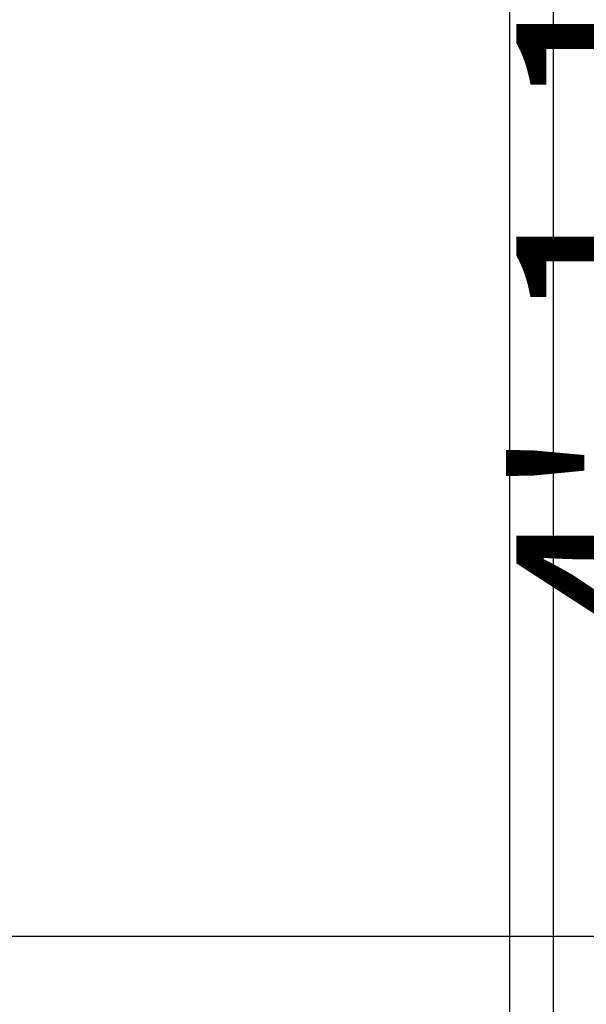
# Model space of a CAD drawing. Units: inches. Extents: x 459864 to 460310, y 324185 to 324787.
# Tile 106 of 112: x 460255 to 460272, y 324281 to 324311. Entities that reach past the tile are written whole.
import ezdxf

# ---------------------------------------------------------------- set-up
doc = ezdxf.new("R2010")
doc.units = ezdxf.units.IN
for name, color, linetype, lineweight in [('A-ANNO-DIMS', 2, 'Continuous', 18), ('C-PROP', 7, 'Continuous', 30), ('L-HRDS', 9, 'Continuous', 18), ('L-SITE-PATT', 252, 'Continuous', 13)]:
    doc.layers.add(name, color=color, linetype=linetype, lineweight=lineweight)
doc.styles.get("Standard").update_dxf_attribs({"font": 'arial.ttf'})
doc.dimstyles.new('ISO-25', dxfattribs={"dimtxt": 6, "dimasz": 2.5, "dimexe": 1.25, "dimexo": 0.625, "dimtad": 1, "dimdec": 1, "dimlunit": 3, "dimtxsty": 'Standard', "dimcen": 2.5, "dimadec": 0, "dimazin": 0, "dimtfac": 1, "dimtdec": 1, "dimtmove": 0, "dimatfit": 3, "dimfxl": 1, "dimarcsym": 0})

# ---------------------------------------------------------------- blocks, each defined once
blk = doc.blocks.new('*D21')
at = {"layer": 'A-ANNO-DIMS', "color": 0, "lineweight": -2, "transparency": 16777216}
for p, q in [((460247.74, 324715.483), (460309.58, 324715.483)), ((460308.33, 324712.983), (460308.33, 324285.983)), ((460247.74, 324283.483), (460309.58, 324283.483))]:
    blk.add_line(p, q, dxfattribs=at)
at = {"layer": 'A-ANNO-DIMS', "color": 0, "transparency": 16777216}
for points in [[(460307.914, 324712.983), (460308.747, 324712.983), (460308.33, 324715.483)], [(460307.914, 324285.983), (460308.747, 324285.983), (460308.33, 324283.483)]]:
    blk.add_solid(points, dxfattribs=at)
at = {"layer": 'Defpoints', "color": 0, "transparency": 16777216}
for p in [(460247.115, 324715.483), (460247.115, 324283.483), (460308.33, 324283.483)]:
    blk.add_point(p, dxfattribs=at)
at = {"layer": 'A-ANNO-DIMS', "color": 0, "transparency": 16777216, "insert": (460304.64, 324499.483), "char_height": 6, "attachment_point": 5, "rotation": 90}
blk.add_mtext("36'", dxfattribs=at)
blk = doc.blocks.new('*D62')
at = {"layer": 'A-ANNO-DIMS', "color": 0, "lineweight": -2, "transparency": 16777216}
for p, q in [((460247.74, 324332.739), (460278.765, 324332.739)), ((460277.515, 324330.239), (460277.515, 324285.983)), ((460247.74, 324283.483), (460278.765, 324283.483))]:
    blk.add_line(p, q, dxfattribs=at)
at = {"layer": 'A-ANNO-DIMS', "color": 0, "transparency": 16777216}
for points in [[(460277.098, 324330.239), (460277.932, 324330.239), (460277.515, 324332.739)], [(460277.098, 324285.983), (460277.932, 324285.983), (460277.515, 324283.483)]]:
    blk.add_solid(points, dxfattribs=at)
at = {"layer": 'Defpoints', "color": 0, "transparency": 16777216}
for p in [(460247.115, 324332.739), (460247.115, 324283.483), (460277.515, 324283.483)]:
    blk.add_point(p, dxfattribs=at)
at = {"layer": 'A-ANNO-DIMS', "color": 0, "transparency": 16777216, "insert": (460273.788, 324308.111), "char_height": 6, "attachment_point": 5, "rotation": 90}
blk.add_mtext('4\'-1 1/2"', dxfattribs=at)
blk = doc.blocks.new('*D65')
at = {"layer": 'A-ANNO-DIMS', "color": 0, "lineweight": -2, "transparency": 16777216}
for p, q in [((460247.74, 324283.483), (460302.765, 324283.483)), ((460301.515, 324280.983), (460301.515, 324197.483)), ((460271.74, 324194.983), (460302.765, 324194.983))]:
    blk.add_line(p, q, dxfattribs=at)
at = {"layer": 'A-ANNO-DIMS', "color": 0, "transparency": 16777216}
for points in [[(460301.098, 324280.983), (460301.932, 324280.983), (460301.515, 324283.483)], [(460301.098, 324197.483), (460301.932, 324197.483), (460301.515, 324194.983)]]:
    blk.add_solid(points, dxfattribs=at)
at = {"layer": 'Defpoints', "color": 0, "transparency": 16777216}
for p in [(460247.115, 324283.483), (460271.115, 324194.983), (460301.515, 324194.983)]:
    blk.add_point(p, dxfattribs=at)
at = {"layer": 'A-ANNO-DIMS', "color": 0, "transparency": 16777216, "insert": (460297.788, 324239.233), "char_height": 6, "attachment_point": 5, "rotation": 90}
blk.add_mtext('7\'-4 1/2"', dxfattribs=at)

msp = doc.modelspace()

# ---------------------------------------------------------------- hatches: boundary and pattern name
at = {"layer": 'L-SITE-PATT'}
h = msp.add_hatch(dxfattribs=at)
h.set_pattern_fill('DOTS', color=256)
h.paths.add_polyline_path([(460269.804, 324283.483), (460247.115, 324283.483), (460121.929, 324283.483), (460121.929, 324252.473), (460117.429, 324252.473), (460110.124, 324252.473), (460110.124, 324243.287), (460080.83, 324243.287), (460080.83, 324252.473), (460061.115, 324252.473), (460061.115, 324251.882), (460077.909, 324251.882), (460077.909, 324199.483), (460080.83, 324199.483), (460080.83, 324207.553), (460110.124, 324207.553), (460110.124, 324199.483), (460110.813, 324199.483), (460262.115, 324199.483), (460269.804, 324199.483)], flags=17)
edge = h.paths.add_edge_path(flags=0)
edge.add_ellipse((460222.59, 324263.813), major_axis=(-8.485, 8.485), ratio=1, start_angle=405, end_angle=495, ccw=False)
edge.add_line((460214.821, 324254.66), (460214.832, 324254.666))
edge.add_ellipse((460222.59, 324263.813), major_axis=(-8.485, 8.485), ratio=1, start_angle=405, end_angle=495, ccw=False)
edge.add_line((460210.759, 324261.781), (460210.768, 324261.787))
edge.add_ellipse((460222.59, 324263.813), major_axis=(-8.485, 8.485), ratio=1, start_angle=405, end_angle=495, ccw=False)
edge.add_ellipse((460222.59, 324263.813), major_axis=(-8.485, 8.485), ratio=1, start_angle=392.754, end_angle=405, ccw=False)
edge.add_ellipse((460222.59, 324263.813), major_axis=(-8.485, 8.485), ratio=1, start_angle=380.9347, end_angle=392.754, ccw=False)
edge.add_line((460211.337, 324267.985), (460211.34, 324267.985))
edge.add_ellipse((460222.59, 324263.813), major_axis=(-8.485, 8.485), ratio=1, start_angle=380.9347, end_angle=392.754, ccw=False)
edge.add_ellipse((460222.59, 324263.813), major_axis=(-8.485, 8.485), ratio=1, start_angle=347.9015, end_angle=380.9347, ccw=False)
edge.add_ellipse((460222.59, 324263.813), major_axis=(-8.485, 8.485), ratio=1, start_angle=327.0619, end_angle=347.9015, ccw=False)
edge.add_ellipse((460222.59, 324263.813), major_axis=(-8.485, 8.485), ratio=1, start_angle=278.3246, end_angle=327.0619, ccw=False)
edge.add_line((460225.158, 324275.536), (460225.158, 324275.535))
edge.add_ellipse((460222.59, 324263.813), major_axis=(-8.485, 8.485), ratio=1, start_angle=278.3246, end_angle=327.0619, ccw=False)
edge.add_ellipse((460222.59, 324263.813), major_axis=(-8.485, 8.485), ratio=1, start_angle=260.6436, end_angle=278.3246, ccw=False)
edge.add_ellipse((460222.59, 324263.813), major_axis=(-8.485, 8.485), ratio=1, start_angle=225, end_angle=260.6436, ccw=False)
edge.add_line((460234.509, 324265.243), (460234.501, 324265.239))
edge.add_ellipse((460222.59, 324263.813), major_axis=(-8.485, 8.485), ratio=1, start_angle=225, end_angle=260.6436, ccw=False)
edge.add_ellipse((460222.59, 324263.813), major_axis=(-8.485, 8.485), ratio=1, start_angle=495, end_angle=585, ccw=False)
edge.add_line((460234.437, 324261.861), (460234.424, 324261.858))
edge.add_ellipse((460222.59, 324263.813), major_axis=(-8.485, 8.485), ratio=1, start_angle=495, end_angle=585, ccw=False)
edge.add_line((460227.95, 324253.067), (460227.946, 324253.083))
edge.add_ellipse((460222.59, 324263.813), major_axis=(-8.485, 8.485), ratio=1, start_angle=495, end_angle=585, ccw=False)
edge.add_line((460226.223, 324252.369), (460226.211, 324252.38))
edge.add_ellipse((460222.59, 324263.813), major_axis=(-8.485, 8.485), ratio=1, start_angle=495, end_angle=585, ccw=False)
h.paths.add_polyline_path([(460219.651, 324254.347), (460218.461, 324253.545), (460218.275, 324254.789), (460219.642, 324256.542), (460219.625, 324260.848), (460216.11, 324257.333), (460214.35, 324256.978), (460215.416, 324259.356), (460212.524, 324258.496), (460213.137, 324259.93), (460218.507, 324263.813), (460222.59, 324263.813), (460222.59, 324267.807), (460218.176, 324272.212), (460219.026, 324274.639), (460222.59, 324272.811), (460222.59, 324275.423), (460223.057, 324274.825), (460222.675, 324273.492), (460225.912, 324267.135), (460219.625, 324260.848)], flags=0)
edge = h.paths.add_edge_path(flags=0)
edge.add_ellipse((460194.576, 324264.046), major_axis=(-8.485, 8.485), ratio=1, start_angle=495, end_angle=585, ccw=False)
edge.add_line((460199.936, 324253.3), (460199.932, 324253.316))
edge.add_ellipse((460194.576, 324264.046), major_axis=(-8.485, 8.485), ratio=1, start_angle=495, end_angle=585, ccw=False)
edge.add_line((460198.208, 324252.603), (460198.196, 324252.613))
edge.add_ellipse((460194.576, 324264.046), major_axis=(-8.485, 8.485), ratio=1, start_angle=495, end_angle=585, ccw=False)
edge.add_ellipse((460194.576, 324264.046), major_axis=(-8.485, 8.485), ratio=1, start_angle=405, end_angle=495, ccw=False)
edge.add_line((460186.806, 324254.893), (460186.817, 324254.899))
edge.add_ellipse((460194.576, 324264.046), major_axis=(-8.485, 8.485), ratio=1, start_angle=405, end_angle=495, ccw=False)
edge.add_line((460182.744, 324262.014), (460182.753, 324262.02))
edge.add_ellipse((460194.576, 324264.046), major_axis=(-8.485, 8.485), ratio=1, start_angle=405, end_angle=495, ccw=False)
edge.add_ellipse((460194.576, 324264.046), major_axis=(-8.485, 8.485), ratio=1, start_angle=392.754, end_angle=405, ccw=False)
edge.add_ellipse((460194.576, 324264.046), major_axis=(-8.485, 8.485), ratio=1, start_angle=380.9347, end_angle=392.754, ccw=False)
edge.add_line((460183.323, 324268.218), (460183.326, 324268.218))
edge.add_ellipse((460194.576, 324264.046), major_axis=(-8.485, 8.485), ratio=1, start_angle=380.9347, end_angle=392.754, ccw=False)
edge.add_ellipse((460194.576, 324264.046), major_axis=(-8.485, 8.485), ratio=1, start_angle=347.9015, end_angle=380.9347, ccw=False)
edge.add_ellipse((460194.576, 324264.046), major_axis=(-8.485, 8.485), ratio=1, start_angle=327.0619, end_angle=347.9015, ccw=False)
edge.add_ellipse((460194.576, 324264.046), major_axis=(-8.485, 8.485), ratio=1, start_angle=278.3246, end_angle=327.0619, ccw=False)
edge.add_line((460197.144, 324275.769), (460197.143, 324275.768))
edge.add_ellipse((460194.576, 324264.046), major_axis=(-8.485, 8.485), ratio=1, start_angle=278.3246, end_angle=327.0619, ccw=False)
edge.add_ellipse((460194.576, 324264.046), major_axis=(-8.485, 8.485), ratio=1, start_angle=260.6436, end_angle=278.3246, ccw=False)
edge.add_ellipse((460194.576, 324264.046), major_axis=(-8.485, 8.485), ratio=1, start_angle=225, end_angle=260.6436, ccw=False)
edge.add_line((460206.494, 324265.476), (460206.487, 324265.473))
edge.add_ellipse((460194.576, 324264.046), major_axis=(-8.485, 8.485), ratio=1, start_angle=225, end_angle=260.6436, ccw=False)
edge.add_ellipse((460194.576, 324264.046), major_axis=(-8.485, 8.485), ratio=1, start_angle=495, end_angle=585, ccw=False)
edge.add_line((460206.422, 324262.094), (460206.409, 324262.091))
h.paths.add_polyline_path([(460191.61, 324261.081), (460191.637, 324254.58), (460190.447, 324253.778), (460190.261, 324255.023), (460191.628, 324256.775), (460191.61, 324261.081), (460188.096, 324257.566), (460186.335, 324257.211), (460187.402, 324259.589), (460184.509, 324258.729), (460185.123, 324260.163), (460190.493, 324264.046), (460194.576, 324264.046), (460194.576, 324268.04), (460190.161, 324272.446), (460191.011, 324274.872), (460194.576, 324273.044), (460194.576, 324275.657), (460195.043, 324275.058), (460194.661, 324273.725), (460197.897, 324267.368)], flags=0)
edge = h.paths.add_edge_path(flags=0)
edge.add_ellipse((460252.912, 324263.578), major_axis=(-8.485, 8.485), ratio=1, start_angle=405, end_angle=495, ccw=False)
edge.add_line((460241.081, 324261.545), (460241.089, 324261.551))
edge.add_ellipse((460252.912, 324263.578), major_axis=(-8.485, 8.485), ratio=1, start_angle=405, end_angle=495, ccw=False)
edge.add_ellipse((460252.912, 324263.578), major_axis=(-8.485, 8.485), ratio=1, start_angle=392.754, end_angle=405, ccw=False)
edge.add_ellipse((460252.912, 324263.578), major_axis=(-8.485, 8.485), ratio=1, start_angle=380.9347, end_angle=392.754, ccw=False)
edge.add_line((460241.659, 324267.749), (460241.662, 324267.749))
edge.add_ellipse((460252.912, 324263.578), major_axis=(-8.485, 8.485), ratio=1, start_angle=380.9347, end_angle=392.754, ccw=False)
edge.add_ellipse((460252.912, 324263.578), major_axis=(-8.485, 8.485), ratio=1, start_angle=347.9015, end_angle=380.9347, ccw=False)
edge.add_ellipse((460252.912, 324263.578), major_axis=(-8.485, 8.485), ratio=1, start_angle=327.0619, end_angle=347.9015, ccw=False)
edge.add_ellipse((460252.912, 324263.578), major_axis=(-8.485, 8.485), ratio=1, start_angle=278.3246, end_angle=327.0619, ccw=False)
edge.add_line((460255.48, 324275.3), (460255.479, 324275.299))
edge.add_ellipse((460252.912, 324263.578), major_axis=(-8.485, 8.485), ratio=1, start_angle=278.3246, end_angle=327.0619, ccw=False)
edge.add_ellipse((460252.912, 324263.578), major_axis=(-8.485, 8.485), ratio=1, start_angle=260.6436, end_angle=278.3246, ccw=False)
edge.add_ellipse((460252.912, 324263.578), major_axis=(-8.485, 8.485), ratio=1, start_angle=225, end_angle=260.6436, ccw=False)
edge.add_line((460264.83, 324265.007), (460264.823, 324265.004))
edge.add_ellipse((460252.912, 324263.578), major_axis=(-8.485, 8.485), ratio=1, start_angle=225, end_angle=260.6436, ccw=False)
edge.add_ellipse((460252.912, 324263.578), major_axis=(-8.485, 8.485), ratio=1, start_angle=495, end_angle=585, ccw=False)
edge.add_line((460264.758, 324261.626), (460264.745, 324261.622))
edge.add_ellipse((460252.912, 324263.578), major_axis=(-8.485, 8.485), ratio=1, start_angle=495, end_angle=585, ccw=False)
edge.add_line((460258.272, 324252.832), (460258.268, 324252.848))
edge.add_ellipse((460252.912, 324263.578), major_axis=(-8.485, 8.485), ratio=1, start_angle=495, end_angle=585, ccw=False)
edge.add_line((460256.545, 324252.134), (460256.533, 324252.144))
edge.add_ellipse((460252.912, 324263.578), major_axis=(-8.485, 8.485), ratio=1, start_angle=495, end_angle=585, ccw=False)
edge.add_ellipse((460252.912, 324263.578), major_axis=(-8.485, 8.485), ratio=1, start_angle=405, end_angle=495, ccw=False)
edge.add_line((460245.143, 324254.424), (460245.153, 324254.43))
h.paths.add_polyline_path([(460244.672, 324256.742), (460245.738, 324259.12), (460242.846, 324258.26), (460243.459, 324259.694), (460248.829, 324263.578), (460252.912, 324263.578), (460252.912, 324267.571), (460248.497, 324271.977), (460249.348, 324274.403), (460252.912, 324272.576), (460252.912, 324275.188), (460253.379, 324274.589), (460252.997, 324273.257), (460256.233, 324266.899), (460249.946, 324260.612), (460249.973, 324254.111), (460248.783, 324253.309), (460248.597, 324254.554), (460249.964, 324256.306), (460249.946, 324260.612), (460246.432, 324257.097)], flags=0)
edge = h.paths.add_edge_path(flags=0)
edge.add_ellipse((460167.439, 324262.833), major_axis=(-8.485, 8.485), ratio=1, start_angle=495, end_angle=585, ccw=False)
edge.add_line((460172.799, 324252.087), (460172.795, 324252.103))
edge.add_ellipse((460167.439, 324262.833), major_axis=(-8.485, 8.485), ratio=1, start_angle=495, end_angle=585, ccw=False)
edge.add_line((460171.071, 324251.389), (460171.059, 324251.399))
edge.add_ellipse((460167.439, 324262.833), major_axis=(-8.485, 8.485), ratio=1, start_angle=495, end_angle=585, ccw=False)
edge.add_ellipse((460167.439, 324262.833), major_axis=(-8.485, 8.485), ratio=1, start_angle=405, end_angle=495, ccw=False)
edge.add_line((460159.669, 324253.679), (460159.68, 324253.685))
edge.add_ellipse((460167.439, 324262.833), major_axis=(-8.485, 8.485), ratio=1, start_angle=405, end_angle=495, ccw=False)
edge.add_line((460155.607, 324260.8), (460155.616, 324260.806))
edge.add_ellipse((460167.439, 324262.833), major_axis=(-8.485, 8.485), ratio=1, start_angle=405, end_angle=495, ccw=False)
edge.add_ellipse((460167.439, 324262.833), major_axis=(-8.485, 8.485), ratio=1, start_angle=392.754, end_angle=405, ccw=False)
edge.add_ellipse((460167.439, 324262.833), major_axis=(-8.485, 8.485), ratio=1, start_angle=380.9347, end_angle=392.754, ccw=False)
edge.add_line((460156.185, 324267.005), (460156.189, 324267.005))
edge.add_ellipse((460167.439, 324262.833), major_axis=(-8.485, 8.485), ratio=1, start_angle=380.9347, end_angle=392.754, ccw=False)
edge.add_ellipse((460167.439, 324262.833), major_axis=(-8.485, 8.485), ratio=1, start_angle=347.9015, end_angle=380.9347, ccw=False)
edge.add_ellipse((460167.439, 324262.833), major_axis=(-8.485, 8.485), ratio=1, start_angle=327.0619, end_angle=347.9015, ccw=False)
edge.add_ellipse((460167.439, 324262.833), major_axis=(-8.485, 8.485), ratio=1, start_angle=278.3246, end_angle=327.0619, ccw=False)
edge.add_line((460170.007, 324274.556), (460170.006, 324274.554))
edge.add_ellipse((460167.439, 324262.833), major_axis=(-8.485, 8.485), ratio=1, start_angle=278.3246, end_angle=327.0619, ccw=False)
edge.add_ellipse((460167.439, 324262.833), major_axis=(-8.485, 8.485), ratio=1, start_angle=260.6436, end_angle=278.3246, ccw=False)
edge.add_ellipse((460167.439, 324262.833), major_axis=(-8.485, 8.485), ratio=1, start_angle=225, end_angle=260.6436, ccw=False)
edge.add_line((460179.357, 324264.262), (460179.35, 324264.259))
edge.add_ellipse((460167.439, 324262.833), major_axis=(-8.485, 8.485), ratio=1, start_angle=225, end_angle=260.6436, ccw=False)
edge.add_ellipse((460167.439, 324262.833), major_axis=(-8.485, 8.485), ratio=1, start_angle=495, end_angle=585, ccw=False)
edge.add_line((460179.285, 324260.881), (460179.272, 324260.877))
h.paths.add_polyline_path([(460164.473, 324259.867), (460164.5, 324253.366), (460163.31, 324252.565), (460163.124, 324253.809), (460164.491, 324255.561), (460164.473, 324259.867), (460160.958, 324256.353), (460159.198, 324255.998), (460160.265, 324258.375), (460157.372, 324257.515), (460157.986, 324258.949), (460163.356, 324262.833), (460167.439, 324262.833), (460167.439, 324266.826), (460163.024, 324271.232), (460163.874, 324273.659), (460167.439, 324271.831), (460167.439, 324274.443), (460167.905, 324273.844), (460167.524, 324272.512), (460170.76, 324266.154)], flags=0)
edge = h.paths.add_edge_path(flags=0)
edge.add_ellipse((460140.758, 324262.37), major_axis=(-8.485, 8.485), ratio=1, start_angle=495, end_angle=585, ccw=False)
edge.add_line((460146.118, 324251.624), (460146.114, 324251.639))
edge.add_ellipse((460140.758, 324262.37), major_axis=(-8.485, 8.485), ratio=1, start_angle=495, end_angle=585, ccw=False)
edge.add_line((460144.391, 324250.926), (460144.379, 324250.936))
edge.add_ellipse((460140.758, 324262.37), major_axis=(-8.485, 8.485), ratio=1, start_angle=495, end_angle=585, ccw=False)
edge.add_ellipse((460140.758, 324262.37), major_axis=(-8.485, 8.485), ratio=1, start_angle=405, end_angle=495, ccw=False)
edge.add_line((460132.989, 324253.216), (460132.999, 324253.222))
edge.add_ellipse((460140.758, 324262.37), major_axis=(-8.485, 8.485), ratio=1, start_angle=405, end_angle=495, ccw=False)
edge.add_line((460128.927, 324260.337), (460128.935, 324260.343))
edge.add_ellipse((460140.758, 324262.37), major_axis=(-8.485, 8.485), ratio=1, start_angle=405, end_angle=495, ccw=False)
edge.add_ellipse((460140.758, 324262.37), major_axis=(-8.485, 8.485), ratio=1, start_angle=392.754, end_angle=405, ccw=False)
edge.add_ellipse((460140.758, 324262.37), major_axis=(-8.485, 8.485), ratio=1, start_angle=380.9347, end_angle=392.754, ccw=False)
edge.add_line((460129.505, 324266.541), (460129.508, 324266.541))
edge.add_ellipse((460140.758, 324262.37), major_axis=(-8.485, 8.485), ratio=1, start_angle=380.9347, end_angle=392.754, ccw=False)
edge.add_ellipse((460140.758, 324262.37), major_axis=(-8.485, 8.485), ratio=1, start_angle=347.9015, end_angle=380.9347, ccw=False)
edge.add_ellipse((460140.758, 324262.37), major_axis=(-8.485, 8.485), ratio=1, start_angle=327.0619, end_angle=347.9015, ccw=False)
edge.add_ellipse((460140.758, 324262.37), major_axis=(-8.485, 8.485), ratio=1, start_angle=278.3246, end_angle=327.0619, ccw=False)
edge.add_line((460143.326, 324274.092), (460143.325, 324274.091))
edge.add_ellipse((460140.758, 324262.37), major_axis=(-8.485, 8.485), ratio=1, start_angle=278.3246, end_angle=327.0619, ccw=False)
edge.add_ellipse((460140.758, 324262.37), major_axis=(-8.485, 8.485), ratio=1, start_angle=260.6436, end_angle=278.3246, ccw=False)
edge.add_ellipse((460140.758, 324262.37), major_axis=(-8.485, 8.485), ratio=1, start_angle=225, end_angle=260.6436, ccw=False)
edge.add_line((460152.677, 324263.799), (460152.669, 324263.796))
edge.add_ellipse((460140.758, 324262.37), major_axis=(-8.485, 8.485), ratio=1, start_angle=225, end_angle=260.6436, ccw=False)
edge.add_ellipse((460140.758, 324262.37), major_axis=(-8.485, 8.485), ratio=1, start_angle=495, end_angle=585, ccw=False)
edge.add_line((460152.604, 324260.418), (460152.592, 324260.414))
h.paths.add_polyline_path([(460137.792, 324259.404), (460137.819, 324252.903), (460136.629, 324252.101), (460136.443, 324253.346), (460137.81, 324255.098), (460137.792, 324259.404), (460134.278, 324255.889), (460132.518, 324255.534), (460133.584, 324257.912), (460130.692, 324257.052), (460131.305, 324258.486), (460136.675, 324262.37), (460140.758, 324262.37), (460140.758, 324266.363), (460136.343, 324270.769), (460137.194, 324273.195), (460140.758, 324271.367), (460140.758, 324273.98), (460141.225, 324273.381), (460140.843, 324272.049), (460144.079, 324265.691)], flags=0)
h.paths.add_polyline_path([(460110.124, 324227.414), (460080.83, 324227.414), (460080.83, 324235.484), (460110.124, 324235.484)], flags=16)
h.paths.add_polyline_path([(460110.124, 324220.797), (460110.124, 324212.727), (460080.83, 324212.727), (460080.83, 324220.797)], flags=16)
h.paths.add_polyline_path([(460269.804, 324283.483), (460247.115, 324283.483), (460121.929, 324283.483), (460121.929, 324252.473), (460117.429, 324252.473), (460110.124, 324252.473), (460110.124, 324243.287), (460080.83, 324243.287), (460080.83, 324252.473), (460061.115, 324252.473), (460061.115, 324251.882), (460077.909, 324251.882), (460077.909, 324199.483), (460080.83, 324199.483), (460080.83, 324207.553), (460110.124, 324207.553), (460110.124, 324199.483), (460262.115, 324199.483), (460269.804, 324199.483)], flags=17)
h.paths.add_polyline_path([(460219.651, 324254.347), (460218.461, 324253.545), (460218.275, 324254.789), (460219.642, 324256.542), (460219.625, 324260.848), (460216.11, 324257.333), (460214.35, 324256.978), (460215.416, 324259.356), (460212.524, 324258.496), (460213.137, 324259.93), (460218.507, 324263.813), (460222.59, 324263.813), (460220.18, 324266.223), (460215.461, 324265.308), (460211.835, 324266.137), (460216.247, 324267.985), (460218.418, 324267.985), (460222.59, 324263.813), (460222.59, 324267.807), (460218.176, 324272.212), (460219.026, 324274.639), (460222.59, 324272.811), (460222.59, 324275.423), (460223.057, 324274.825), (460222.675, 324273.492), (460225.912, 324267.135), (460222.59, 324263.813), (460231.383, 324263.813), (460228.485, 324262.488), (460224.425, 324261.978), (460228.68, 324257.724), (460228.966, 324254.791), (460227.142, 324256.537), (460227.542, 324254.819), (460227.333, 324253.614), (460222.59, 324259.985), (460222.59, 324255.497), (460221.377, 324256.541), (460220.576, 324261.799), (460219.625, 324260.848)], flags=0)
h.paths.add_polyline_path([(460199.127, 324256.77), (460199.528, 324255.052), (460199.319, 324253.848), (460194.576, 324260.218), (460194.576, 324255.73), (460193.363, 324256.774), (460192.561, 324262.032), (460191.61, 324261.081), (460191.637, 324254.58), (460190.447, 324253.778), (460190.261, 324255.023), (460191.628, 324256.775), (460191.61, 324261.081), (460188.096, 324257.566), (460186.335, 324257.211), (460187.402, 324259.589), (460184.509, 324258.729), (460185.123, 324260.163), (460190.493, 324264.046), (460194.576, 324264.046), (460192.166, 324266.456), (460187.446, 324265.541), (460183.82, 324266.37), (460188.232, 324268.218), (460190.404, 324268.218), (460194.576, 324264.046), (460194.576, 324268.04), (460190.161, 324272.446), (460191.011, 324274.872), (460194.576, 324273.044), (460194.576, 324275.657), (460195.043, 324275.058), (460194.661, 324273.725), (460197.897, 324267.368), (460194.576, 324264.046), (460203.368, 324264.046), (460200.47, 324262.721), (460196.411, 324262.212), (460200.665, 324257.957), (460200.951, 324255.024)], flags=0)
h.paths.add_polyline_path([(460244.672, 324256.742), (460245.738, 324259.12), (460242.846, 324258.26), (460243.459, 324259.694), (460248.829, 324263.578), (460252.912, 324263.578), (460250.502, 324265.987), (460245.783, 324265.072), (460242.156, 324265.901), (460246.568, 324267.749), (460248.74, 324267.749), (460252.912, 324263.578), (460252.912, 324267.571), (460248.497, 324271.977), (460249.348, 324274.403), (460252.912, 324272.576), (460252.912, 324275.188), (460253.379, 324274.589), (460252.997, 324273.257), (460256.233, 324266.899), (460252.912, 324263.578), (460261.705, 324263.578), (460258.806, 324262.252), (460254.747, 324261.743), (460259.002, 324257.488), (460259.288, 324254.555), (460257.463, 324256.301), (460257.864, 324254.583), (460257.655, 324253.379), (460252.912, 324259.749), (460252.912, 324255.261), (460251.699, 324256.305), (460250.897, 324261.563), (460249.946, 324260.612), (460249.973, 324254.111), (460248.783, 324253.309), (460248.597, 324254.554), (460249.964, 324256.306), (460249.946, 324260.612), (460246.432, 324257.097)], flags=0)
h.paths.add_polyline_path([(460173.528, 324256.743), (460173.814, 324253.811), (460171.99, 324255.556), (460172.39, 324253.838), (460172.182, 324252.634), (460167.439, 324259.004), (460167.439, 324254.516), (460166.226, 324255.56), (460165.424, 324260.818), (460164.473, 324259.867), (460164.5, 324253.366), (460163.31, 324252.565), (460163.124, 324253.809), (460164.491, 324255.561), (460164.473, 324259.867), (460160.958, 324256.353), (460159.198, 324255.998), (460160.265, 324258.375), (460157.372, 324257.515), (460157.986, 324258.949), (460163.356, 324262.833), (460167.439, 324262.833), (460165.029, 324265.243), (460160.309, 324264.327), (460156.683, 324265.156), (460161.095, 324267.005), (460163.267, 324267.005), (460167.439, 324262.833), (460167.439, 324266.826), (460163.024, 324271.232), (460163.874, 324273.659), (460167.439, 324271.831), (460167.439, 324274.443), (460167.905, 324273.844), (460167.524, 324272.512), (460170.76, 324266.154), (460167.439, 324262.833), (460176.231, 324262.833), (460173.333, 324261.507), (460169.274, 324260.998)], flags=0)
h.paths.add_polyline_path([(460146.848, 324256.28), (460147.134, 324253.347), (460145.31, 324255.093), (460145.71, 324253.375), (460145.501, 324252.171), (460140.758, 324258.541), (460140.758, 324254.053), (460139.545, 324255.097), (460138.744, 324260.355), (460137.792, 324259.404), (460137.819, 324252.903), (460136.629, 324252.101), (460136.443, 324253.346), (460137.81, 324255.098), (460137.792, 324259.404), (460134.278, 324255.889), (460132.518, 324255.534), (460133.584, 324257.912), (460130.692, 324257.052), (460131.305, 324258.486), (460136.675, 324262.37), (460140.758, 324262.37), (460138.348, 324264.779), (460133.629, 324263.864), (460130.002, 324264.693), (460134.414, 324266.541), (460136.586, 324266.541), (460140.758, 324262.37), (460140.758, 324266.363), (460136.343, 324270.769), (460137.194, 324273.195), (460140.758, 324271.367), (460140.758, 324273.98), (460141.225, 324273.381), (460140.843, 324272.049), (460144.079, 324265.691), (460140.758, 324262.37), (460149.551, 324262.37), (460146.653, 324261.044), (460142.593, 324260.535)], flags=0)
edge = h.paths.add_edge_path()
edge.add_line((460269.804, 324272.549), (460260.881, 324272.549))
edge.add_ellipse((460252.912, 324263.578), major_axis=(-8.485, 8.485), ratio=1, start_angle=260.6436, end_angle=273.3846, ccw=False)
edge.add_line((460262.283, 324271.092), (460262.261, 324271.091))
edge.add_ellipse((460252.912, 324263.578), major_axis=(-8.485, 8.485), ratio=1, start_angle=260.6436, end_angle=273.3846, ccw=False)
edge.add_ellipse((460252.912, 324263.578), major_axis=(-8.485, 8.485), ratio=1, start_angle=225, end_angle=260.6436, ccw=False)
edge.add_line((460263.609, 324269.063), (460263.572, 324269.058))
edge.add_ellipse((460252.912, 324263.578), major_axis=(-8.485, 8.485), ratio=1, start_angle=225, end_angle=260.6436, ccw=False)
edge.add_line((460264.615, 324266.306), (460264.585, 324266.305))
edge.add_ellipse((460252.912, 324263.578), major_axis=(-8.485, 8.485), ratio=1, start_angle=225, end_angle=260.6436, ccw=False)
edge.add_line((460264.83, 324265.007), (460264.823, 324265.004))
edge.add_ellipse((460252.912, 324263.578), major_axis=(-8.485, 8.485), ratio=1, start_angle=225, end_angle=260.6436, ccw=False)
edge.add_ellipse((460252.912, 324263.578), major_axis=(-8.485, 8.485), ratio=1, start_angle=495, end_angle=585, ccw=False)
edge.add_line((460264.758, 324261.626), (460264.745, 324261.622))
edge.add_ellipse((460252.912, 324263.578), major_axis=(-8.485, 8.485), ratio=1, start_angle=495, end_angle=585, ccw=False)
edge.add_line((460263.442, 324257.739), (460263.389, 324257.779))
edge.add_ellipse((460252.912, 324263.578), major_axis=(-8.485, 8.485), ratio=1, start_angle=495, end_angle=585, ccw=False)
edge.add_line((460258.128, 324252.744), (460258.102, 324252.779))
edge.add_ellipse((460252.912, 324263.578), major_axis=(-8.485, 8.485), ratio=1, start_angle=495, end_angle=585, ccw=False)
edge.add_line((460256.545, 324252.134), (460256.533, 324252.144))
edge.add_ellipse((460252.912, 324263.578), major_axis=(-8.485, 8.485), ratio=1, start_angle=495, end_angle=585, ccw=False)
edge.add_ellipse((460252.912, 324263.578), major_axis=(-8.485, 8.485), ratio=1, start_angle=405, end_angle=495, ccw=False)
edge.add_line((460250.594, 324251.78), (460250.605, 324251.82))
edge.add_ellipse((460252.912, 324263.578), major_axis=(-8.485, 8.485), ratio=1, start_angle=405, end_angle=495, ccw=False)
edge.add_line((460245.143, 324254.424), (460245.153, 324254.43))
edge.add_ellipse((460252.912, 324263.578), major_axis=(-8.485, 8.485), ratio=1, start_angle=405, end_angle=495, ccw=False)
edge.add_line((460243.525, 324256.059), (460243.56, 324256.091))
edge.add_ellipse((460252.912, 324263.578), major_axis=(-8.485, 8.485), ratio=1, start_angle=405, end_angle=495, ccw=False)
edge.add_line((460241.44, 324259.893), (460241.522, 324259.896))
edge.add_ellipse((460252.912, 324263.578), major_axis=(-8.485, 8.485), ratio=1, start_angle=405, end_angle=495, ccw=False)
edge.add_line((460241.081, 324261.545), (460241.089, 324261.551))
edge.add_ellipse((460252.912, 324263.578), major_axis=(-8.485, 8.485), ratio=1, start_angle=405, end_angle=495, ccw=False)
edge.add_ellipse((460252.912, 324263.578), major_axis=(-8.485, 8.485), ratio=1, start_angle=392.754, end_angle=405, ccw=False)
edge.add_line((460241.05, 324265.438), (460241.063, 324265.443))
edge.add_ellipse((460252.912, 324263.578), major_axis=(-8.485, 8.485), ratio=1, start_angle=392.754, end_angle=405, ccw=False)
edge.add_ellipse((460252.912, 324263.578), major_axis=(-8.485, 8.485), ratio=1, start_angle=380.9347, end_angle=392.754, ccw=False)
edge.add_line((460241.452, 324267.176), (460241.469, 324267.171))
edge.add_ellipse((460252.912, 324263.578), major_axis=(-8.485, 8.485), ratio=1, start_angle=380.9347, end_angle=392.754, ccw=False)
edge.add_line((460241.659, 324267.749), (460241.662, 324267.749))
edge.add_ellipse((460252.912, 324263.578), major_axis=(-8.485, 8.485), ratio=1, start_angle=380.9347, end_angle=392.754, ccw=False)
edge.add_ellipse((460252.912, 324263.578), major_axis=(-8.485, 8.485), ratio=1, start_angle=356.6154, end_angle=380.9347, ccw=False)
edge.add_line((460244.88, 324272.488), (460244.713, 324272.549))
edge.add_line((460244.713, 324272.549), (460230.817, 324272.549))
edge.add_ellipse((460222.59, 324263.813), major_axis=(-8.485, 8.485), ratio=1, start_angle=260.6436, end_angle=271.7178, ccw=False)
edge.add_ellipse((460222.59, 324263.813), major_axis=(-8.485, 8.485), ratio=1, start_angle=225, end_angle=260.6436, ccw=False)
edge.add_line((460233.287, 324269.299), (460233.25, 324269.294))
edge.add_ellipse((460222.59, 324263.813), major_axis=(-8.485, 8.485), ratio=1, start_angle=225, end_angle=260.6436, ccw=False)
edge.add_line((460234.294, 324266.541), (460234.264, 324266.541))
edge.add_ellipse((460222.59, 324263.813), major_axis=(-8.485, 8.485), ratio=1, start_angle=225, end_angle=260.6436, ccw=False)
edge.add_line((460234.509, 324265.243), (460234.501, 324265.239))
edge.add_ellipse((460222.59, 324263.813), major_axis=(-8.485, 8.485), ratio=1, start_angle=225, end_angle=260.6436, ccw=False)
edge.add_ellipse((460222.59, 324263.813), major_axis=(-8.485, 8.485), ratio=1, start_angle=495, end_angle=585, ccw=False)
edge.add_line((460234.437, 324261.861), (460234.424, 324261.858))
edge.add_ellipse((460222.59, 324263.813), major_axis=(-8.485, 8.485), ratio=1, start_angle=495, end_angle=585, ccw=False)
edge.add_line((460233.121, 324257.975), (460233.068, 324258.015))
edge.add_ellipse((460222.59, 324263.813), major_axis=(-8.485, 8.485), ratio=1, start_angle=495, end_angle=585, ccw=False)
edge.add_line((460227.806, 324252.979), (460227.78, 324253.014))
edge.add_ellipse((460222.59, 324263.813), major_axis=(-8.485, 8.485), ratio=1, start_angle=495, end_angle=585, ccw=False)
edge.add_line((460226.223, 324252.369), (460226.211, 324252.38))
edge.add_ellipse((460222.59, 324263.813), major_axis=(-8.485, 8.485), ratio=1, start_angle=495, end_angle=585, ccw=False)
edge.add_ellipse((460222.59, 324263.813), major_axis=(-8.485, 8.485), ratio=1, start_angle=405, end_angle=495, ccw=False)
edge.add_line((460220.272, 324252.016), (460220.283, 324252.055))
edge.add_ellipse((460222.59, 324263.813), major_axis=(-8.485, 8.485), ratio=1, start_angle=405, end_angle=495, ccw=False)
edge.add_line((460214.821, 324254.66), (460214.832, 324254.666))
edge.add_ellipse((460222.59, 324263.813), major_axis=(-8.485, 8.485), ratio=1, start_angle=405, end_angle=495, ccw=False)
edge.add_line((460213.203, 324256.295), (460213.239, 324256.327))
edge.add_ellipse((460222.59, 324263.813), major_axis=(-8.485, 8.485), ratio=1, start_angle=405, end_angle=495, ccw=False)
edge.add_line((460211.118, 324260.128), (460211.201, 324260.131))
edge.add_ellipse((460222.59, 324263.813), major_axis=(-8.485, 8.485), ratio=1, start_angle=405, end_angle=495, ccw=False)
edge.add_line((460210.759, 324261.781), (460210.768, 324261.787))
edge.add_ellipse((460222.59, 324263.813), major_axis=(-8.485, 8.485), ratio=1, start_angle=405, end_angle=495, ccw=False)
edge.add_ellipse((460222.59, 324263.813), major_axis=(-8.485, 8.485), ratio=1, start_angle=392.754, end_angle=405, ccw=False)
edge.add_line((460210.729, 324265.673), (460210.741, 324265.678))
edge.add_ellipse((460222.59, 324263.813), major_axis=(-8.485, 8.485), ratio=1, start_angle=392.754, end_angle=405, ccw=False)
edge.add_ellipse((460222.59, 324263.813), major_axis=(-8.485, 8.485), ratio=1, start_angle=380.9347, end_angle=392.754, ccw=False)
edge.add_line((460211.13, 324267.412), (460211.147, 324267.407))
edge.add_ellipse((460222.59, 324263.813), major_axis=(-8.485, 8.485), ratio=1, start_angle=380.9347, end_angle=392.754, ccw=False)
edge.add_line((460211.337, 324267.985), (460211.34, 324267.985))
edge.add_ellipse((460222.59, 324263.813), major_axis=(-8.485, 8.485), ratio=1, start_angle=380.9347, end_angle=392.754, ccw=False)
edge.add_ellipse((460222.59, 324263.813), major_axis=(-8.485, 8.485), ratio=1, start_angle=358.2822, end_angle=380.9347, ccw=False)
edge.add_line((460213.705, 324271.902), (460213.709, 324271.869))
edge.add_ellipse((460222.59, 324263.813), major_axis=(-8.485, 8.485), ratio=1, start_angle=358.2822, end_angle=380.9347, ccw=False)
edge.add_line((460214.363, 324272.549), (460203.078, 324272.549))
edge.add_line((460203.078, 324272.549), (460203.06, 324272.531))
edge.add_ellipse((460194.576, 324264.046), major_axis=(-8.485, 8.485), ratio=1, start_angle=260.6436, end_angle=270.1168, ccw=False)
edge.add_line((460203.957, 324271.561), (460203.921, 324271.56))
edge.add_ellipse((460194.576, 324264.046), major_axis=(-8.485, 8.485), ratio=1, start_angle=260.6436, end_angle=270.1168, ccw=False)
edge.add_ellipse((460194.576, 324264.046), major_axis=(-8.485, 8.485), ratio=1, start_angle=225, end_angle=260.6436, ccw=False)
edge.add_line((460205.272, 324269.532), (460205.235, 324269.527))
edge.add_ellipse((460194.576, 324264.046), major_axis=(-8.485, 8.485), ratio=1, start_angle=225, end_angle=260.6436, ccw=False)
edge.add_line((460206.279, 324266.774), (460206.249, 324266.774))
edge.add_ellipse((460194.576, 324264.046), major_axis=(-8.485, 8.485), ratio=1, start_angle=225, end_angle=260.6436, ccw=False)
edge.add_line((460206.494, 324265.476), (460206.487, 324265.473))
edge.add_ellipse((460194.576, 324264.046), major_axis=(-8.485, 8.485), ratio=1, start_angle=225, end_angle=260.6436, ccw=False)
edge.add_ellipse((460194.576, 324264.046), major_axis=(-8.485, 8.485), ratio=1, start_angle=495, end_angle=585, ccw=False)
edge.add_line((460206.422, 324262.094), (460206.409, 324262.091))
edge.add_ellipse((460194.576, 324264.046), major_axis=(-8.485, 8.485), ratio=1, start_angle=495, end_angle=585, ccw=False)
edge.add_line((460205.106, 324258.208), (460205.053, 324258.248))
edge.add_ellipse((460194.576, 324264.046), major_axis=(-8.485, 8.485), ratio=1, start_angle=495, end_angle=585, ccw=False)
edge.add_line((460199.792, 324253.212), (460199.766, 324253.248))
edge.add_ellipse((460194.576, 324264.046), major_axis=(-8.485, 8.485), ratio=1, start_angle=495, end_angle=585, ccw=False)
edge.add_line((460198.208, 324252.603), (460198.196, 324252.613))
edge.add_ellipse((460194.576, 324264.046), major_axis=(-8.485, 8.485), ratio=1, start_angle=495, end_angle=585, ccw=False)
edge.add_ellipse((460194.576, 324264.046), major_axis=(-8.485, 8.485), ratio=1, start_angle=405, end_angle=495, ccw=False)
edge.add_line((460192.258, 324252.249), (460192.268, 324252.289))
edge.add_ellipse((460194.576, 324264.046), major_axis=(-8.485, 8.485), ratio=1, start_angle=405, end_angle=495, ccw=False)
edge.add_line((460186.806, 324254.893), (460186.817, 324254.899))
edge.add_ellipse((460194.576, 324264.046), major_axis=(-8.485, 8.485), ratio=1, start_angle=405, end_angle=495, ccw=False)
edge.add_line((460185.188, 324256.528), (460185.224, 324256.56))
edge.add_ellipse((460194.576, 324264.046), major_axis=(-8.485, 8.485), ratio=1, start_angle=405, end_angle=495, ccw=False)
edge.add_line((460183.104, 324260.362), (460183.186, 324260.365))
edge.add_ellipse((460194.576, 324264.046), major_axis=(-8.485, 8.485), ratio=1, start_angle=405, end_angle=495, ccw=False)
edge.add_line((460182.744, 324262.014), (460182.753, 324262.02))
edge.add_ellipse((460194.576, 324264.046), major_axis=(-8.485, 8.485), ratio=1, start_angle=405, end_angle=495, ccw=False)
edge.add_ellipse((460194.576, 324264.046), major_axis=(-8.485, 8.485), ratio=1, start_angle=392.754, end_angle=405, ccw=False)
edge.add_line((460182.714, 324265.906), (460182.726, 324265.912))
edge.add_ellipse((460194.576, 324264.046), major_axis=(-8.485, 8.485), ratio=1, start_angle=392.754, end_angle=405, ccw=False)
edge.add_ellipse((460194.576, 324264.046), major_axis=(-8.485, 8.485), ratio=1, start_angle=380.9347, end_angle=392.754, ccw=False)
edge.add_line((460183.116, 324267.645), (460183.133, 324267.64))
edge.add_ellipse((460194.576, 324264.046), major_axis=(-8.485, 8.485), ratio=1, start_angle=380.9347, end_angle=392.754, ccw=False)
edge.add_line((460183.323, 324268.218), (460183.326, 324268.218))
edge.add_ellipse((460194.576, 324264.046), major_axis=(-8.485, 8.485), ratio=1, start_angle=380.9347, end_angle=392.754, ccw=False)
edge.add_ellipse((460194.576, 324264.046), major_axis=(-8.485, 8.485), ratio=1, start_angle=359.8832, end_angle=380.9347, ccw=False)
edge.add_line((460184.491, 324270.611), (460184.553, 324270.611))
edge.add_ellipse((460194.576, 324264.046), major_axis=(-8.485, 8.485), ratio=1, start_angle=359.8832, end_angle=380.9347, ccw=False)
edge.add_line((460185.346, 324271.76), (460185.379, 324271.728))
edge.add_ellipse((460194.576, 324264.046), major_axis=(-8.485, 8.485), ratio=1, start_angle=359.8832, end_angle=380.9347, ccw=False)
edge.add_line((460185.697, 324272.086), (460185.633, 324272.549))
edge.add_line((460185.633, 324272.549), (460174.683, 324272.549))
edge.add_line((460174.683, 324272.549), (460174.606, 324272.457))
edge.add_ellipse((460167.439, 324262.833), major_axis=(-8.485, 8.485), ratio=1, start_angle=260.6436, end_angle=278.3246, ccw=False)
edge.add_ellipse((460167.439, 324262.833), major_axis=(-8.485, 8.485), ratio=1, start_angle=225, end_angle=260.6436, ccw=False)
edge.add_line((460178.135, 324268.318), (460178.098, 324268.313))
edge.add_ellipse((460167.439, 324262.833), major_axis=(-8.485, 8.485), ratio=1, start_angle=225, end_angle=260.6436, ccw=False)
edge.add_line((460179.142, 324265.561), (460179.112, 324265.56))
edge.add_ellipse((460167.439, 324262.833), major_axis=(-8.485, 8.485), ratio=1, start_angle=225, end_angle=260.6436, ccw=False)
edge.add_line((460179.357, 324264.262), (460179.35, 324264.259))
edge.add_ellipse((460167.439, 324262.833), major_axis=(-8.485, 8.485), ratio=1, start_angle=225, end_angle=260.6436, ccw=False)
edge.add_ellipse((460167.439, 324262.833), major_axis=(-8.485, 8.485), ratio=1, start_angle=495, end_angle=585, ccw=False)
edge.add_line((460179.285, 324260.881), (460179.272, 324260.877))
edge.add_ellipse((460167.439, 324262.833), major_axis=(-8.485, 8.485), ratio=1, start_angle=495, end_angle=585, ccw=False)
edge.add_line((460177.969, 324256.994), (460177.916, 324257.034))
edge.add_ellipse((460167.439, 324262.833), major_axis=(-8.485, 8.485), ratio=1, start_angle=495, end_angle=585, ccw=False)
edge.add_line((460172.655, 324251.999), (460172.629, 324252.034))
edge.add_ellipse((460167.439, 324262.833), major_axis=(-8.485, 8.485), ratio=1, start_angle=495, end_angle=585, ccw=False)
edge.add_line((460171.071, 324251.389), (460171.059, 324251.399))
edge.add_ellipse((460167.439, 324262.833), major_axis=(-8.485, 8.485), ratio=1, start_angle=495, end_angle=585, ccw=False)
edge.add_ellipse((460167.439, 324262.833), major_axis=(-8.485, 8.485), ratio=1, start_angle=405, end_angle=495, ccw=False)
edge.add_line((460165.121, 324251.036), (460165.131, 324251.075))
edge.add_ellipse((460167.439, 324262.833), major_axis=(-8.485, 8.485), ratio=1, start_angle=405, end_angle=495, ccw=False)
edge.add_line((460159.669, 324253.679), (460159.68, 324253.685))
edge.add_ellipse((460167.439, 324262.833), major_axis=(-8.485, 8.485), ratio=1, start_angle=405, end_angle=495, ccw=False)
edge.add_line((460158.051, 324255.314), (460158.087, 324255.347))
edge.add_ellipse((460167.439, 324262.833), major_axis=(-8.485, 8.485), ratio=1, start_angle=405, end_angle=495, ccw=False)
edge.add_line((460155.967, 324259.148), (460156.049, 324259.151))
edge.add_ellipse((460167.439, 324262.833), major_axis=(-8.485, 8.485), ratio=1, start_angle=405, end_angle=495, ccw=False)
edge.add_line((460155.607, 324260.8), (460155.616, 324260.806))
edge.add_ellipse((460167.439, 324262.833), major_axis=(-8.485, 8.485), ratio=1, start_angle=405, end_angle=495, ccw=False)
edge.add_ellipse((460167.439, 324262.833), major_axis=(-8.485, 8.485), ratio=1, start_angle=392.754, end_angle=405, ccw=False)
edge.add_line((460155.577, 324264.693), (460155.589, 324264.698))
edge.add_ellipse((460167.439, 324262.833), major_axis=(-8.485, 8.485), ratio=1, start_angle=392.754, end_angle=405, ccw=False)
edge.add_ellipse((460167.439, 324262.833), major_axis=(-8.485, 8.485), ratio=1, start_angle=380.9347, end_angle=392.754, ccw=False)
edge.add_line((460155.979, 324266.432), (460155.996, 324266.426))
edge.add_ellipse((460167.439, 324262.833), major_axis=(-8.485, 8.485), ratio=1, start_angle=380.9347, end_angle=392.754, ccw=False)
edge.add_line((460156.185, 324267.005), (460156.189, 324267.005))
edge.add_ellipse((460167.439, 324262.833), major_axis=(-8.485, 8.485), ratio=1, start_angle=380.9347, end_angle=392.754, ccw=False)
edge.add_ellipse((460167.439, 324262.833), major_axis=(-8.485, 8.485), ratio=1, start_angle=350.9345, end_angle=380.9347, ccw=False)
edge.add_line((460157.363, 324269.397), (460157.414, 324269.397))
edge.add_ellipse((460167.439, 324262.833), major_axis=(-8.485, 8.485), ratio=1, start_angle=350.9345, end_angle=380.9347, ccw=False)
edge.add_line((460158.221, 324270.535), (460158.236, 324270.519))
edge.add_ellipse((460167.439, 324262.833), major_axis=(-8.485, 8.485), ratio=1, start_angle=350.9345, end_angle=380.9347, ccw=False)
edge.add_line((460159.379, 324271.753), (460159.419, 324271.738))
edge.add_ellipse((460167.439, 324262.833), major_axis=(-8.485, 8.485), ratio=1, start_angle=350.9345, end_angle=380.9347, ccw=False)
edge.add_line((460160.396, 324272.549), (460147.112, 324272.549))
edge.add_ellipse((460140.758, 324262.37), major_axis=(-8.485, 8.485), ratio=1, start_angle=278.3246, end_angle=283.0261, ccw=False)
edge.add_ellipse((460140.758, 324262.37), major_axis=(-8.485, 8.485), ratio=1, start_angle=260.6436, end_angle=278.3246, ccw=False)
edge.add_ellipse((460140.758, 324262.37), major_axis=(-8.485, 8.485), ratio=1, start_angle=225, end_angle=260.6436, ccw=False)
edge.add_line((460151.455, 324267.855), (460151.418, 324267.85))
edge.add_ellipse((460140.758, 324262.37), major_axis=(-8.485, 8.485), ratio=1, start_angle=225, end_angle=260.6436, ccw=False)
edge.add_line((460152.462, 324265.098), (460152.431, 324265.097))
edge.add_ellipse((460140.758, 324262.37), major_axis=(-8.485, 8.485), ratio=1, start_angle=225, end_angle=260.6436, ccw=False)
edge.add_line((460152.677, 324263.799), (460152.669, 324263.796))
edge.add_ellipse((460140.758, 324262.37), major_axis=(-8.485, 8.485), ratio=1, start_angle=225, end_angle=260.6436, ccw=False)
edge.add_ellipse((460140.758, 324262.37), major_axis=(-8.485, 8.485), ratio=1, start_angle=495, end_angle=585, ccw=False)
edge.add_line((460152.604, 324260.418), (460152.592, 324260.414))
edge.add_ellipse((460140.758, 324262.37), major_axis=(-8.485, 8.485), ratio=1, start_angle=495, end_angle=585, ccw=False)
edge.add_line((460151.288, 324256.531), (460151.235, 324256.571))
edge.add_ellipse((460140.758, 324262.37), major_axis=(-8.485, 8.485), ratio=1, start_angle=495, end_angle=585, ccw=False)
edge.add_line((460145.974, 324251.535), (460145.948, 324251.571))
edge.add_ellipse((460140.758, 324262.37), major_axis=(-8.485, 8.485), ratio=1, start_angle=495, end_angle=585, ccw=False)
edge.add_line((460144.391, 324250.926), (460144.379, 324250.936))
edge.add_ellipse((460140.758, 324262.37), major_axis=(-8.485, 8.485), ratio=1, start_angle=495, end_angle=585, ccw=False)
edge.add_ellipse((460140.758, 324262.37), major_axis=(-8.485, 8.485), ratio=1, start_angle=405, end_angle=495, ccw=False)
edge.add_line((460138.44, 324250.572), (460138.451, 324250.612))
edge.add_ellipse((460140.758, 324262.37), major_axis=(-8.485, 8.485), ratio=1, start_angle=405, end_angle=495, ccw=False)
edge.add_line((460132.989, 324253.216), (460132.999, 324253.222))
edge.add_ellipse((460140.758, 324262.37), major_axis=(-8.485, 8.485), ratio=1, start_angle=405, end_angle=495, ccw=False)
edge.add_line((460131.371, 324254.851), (460131.406, 324254.883))
edge.add_ellipse((460140.758, 324262.37), major_axis=(-8.485, 8.485), ratio=1, start_angle=405, end_angle=495, ccw=False)
edge.add_line((460129.286, 324258.685), (460129.369, 324258.688))
edge.add_ellipse((460140.758, 324262.37), major_axis=(-8.485, 8.485), ratio=1, start_angle=405, end_angle=495, ccw=False)
edge.add_line((460128.927, 324260.337), (460128.935, 324260.343))
edge.add_ellipse((460140.758, 324262.37), major_axis=(-8.485, 8.485), ratio=1, start_angle=405, end_angle=495, ccw=False)
edge.add_ellipse((460140.758, 324262.37), major_axis=(-8.485, 8.485), ratio=1, start_angle=392.754, end_angle=405, ccw=False)
edge.add_line((460128.896, 324264.23), (460128.909, 324264.235))
edge.add_ellipse((460140.758, 324262.37), major_axis=(-8.485, 8.485), ratio=1, start_angle=392.754, end_angle=405, ccw=False)
edge.add_ellipse((460140.758, 324262.37), major_axis=(-8.485, 8.485), ratio=1, start_angle=380.9347, end_angle=392.754, ccw=False)
edge.add_line((460129.298, 324265.968), (460129.315, 324265.963))
edge.add_ellipse((460140.758, 324262.37), major_axis=(-8.485, 8.485), ratio=1, start_angle=380.9347, end_angle=392.754, ccw=False)
edge.add_line((460129.505, 324266.541), (460129.508, 324266.541))
edge.add_ellipse((460140.758, 324262.37), major_axis=(-8.485, 8.485), ratio=1, start_angle=380.9347, end_angle=392.754, ccw=False)
edge.add_ellipse((460140.758, 324262.37), major_axis=(-8.485, 8.485), ratio=1, start_angle=347.9015, end_angle=380.9347, ccw=False)
edge.add_line((460130.697, 324268.934), (460130.727, 324268.934))
edge.add_ellipse((460140.758, 324262.37), major_axis=(-8.485, 8.485), ratio=1, start_angle=347.9015, end_angle=380.9347, ccw=False)
edge.add_line((460131.869, 324270.48), (460131.879, 324270.413))
edge.add_ellipse((460140.758, 324262.37), major_axis=(-8.485, 8.485), ratio=1, start_angle=347.9015, end_angle=380.9347, ccw=False)
edge.add_line((460132.734, 324271.277), (460132.705, 324271.287))
edge.add_ellipse((460140.758, 324262.37), major_axis=(-8.485, 8.485), ratio=1, start_angle=347.9015, end_angle=380.9347, ccw=False)
edge.add_line((460134.24, 324272.445), (460134.204, 324272.549))
edge.add_line((460134.204, 324272.549), (460121.929, 324272.549))
edge.add_line((460121.929, 324272.549), (460121.929, 324252.473))
edge.add_line((460121.929, 324252.473), (460117.429, 324252.473))
edge.add_line((460117.429, 324252.473), (460110.124, 324252.473))
edge.add_line((460110.124, 324252.473), (460110.124, 324243.287))
edge.add_line((460110.124, 324243.287), (460080.83, 324243.287))
edge.add_line((460080.83, 324243.287), (460080.83, 324252.473))
edge.add_line((460080.83, 324252.473), (460061.115, 324252.473))
edge.add_line((460061.115, 324252.473), (460061.115, 324251.882))
edge.add_line((460061.115, 324251.882), (460077.909, 324251.882))
edge.add_line((460077.909, 324251.882), (460077.909, 324199.483))
edge.add_line((460077.909, 324199.483), (460080.83, 324199.483))
edge.add_line((460080.83, 324199.483), (460080.83, 324207.553))
edge.add_line((460080.83, 324207.553), (460110.124, 324207.553))
edge.add_line((460110.124, 324207.553), (460110.124, 324199.483))
edge.add_line((460110.124, 324199.483), (460110.813, 324199.483))
edge.add_line((460110.813, 324199.483), (460262.115, 324199.483))
edge.add_line((460262.115, 324199.483), (460269.804, 324199.483))
edge.add_line((460269.804, 324199.483), (460269.804, 324272.549))

# ---------------------------------------------------------------- linework, layer by layer
at = {"layer": 'C-PROP'}
for p, q in [((460269.804, 324466.483), (460269.804, 324199.483)), ((460271.115, 324466.483), (460271.115, 324194.947))]:
    msp.add_line(p, q, dxfattribs=at)
at = {"layer": 'L-HRDS'}
msp.add_line((460247.115, 324283.483), (460271.115, 324283.483), dxfattribs=at)

# ---------------------------------------------------------------- dimensions: what is measured, and where the dimension line sits
at = {"layer": 'A-ANNO-DIMS'}
for base, p1, p2, angle, override, picture, middle in [((460308.33, 324283.483), (460247.115, 324715.483), (460247.115, 324283.483), 90, {"dimclrd": 0, "dimclre": 0, "dimclrt": 0}, '*D21', (460304.64, 324499.483)), ((460277.515, 324283.483), (460247.115, 324332.739), (460247.115, 324283.483), 270, {"dimdec": 1, "dimlfac": 1, "dimrnd": 0, "dimzin": 1, "dimdsep": 46, "dimlunit": 4, "dimfrac": 2}, '*D62', (460273.788, 324308.111)), ((460301.515, 324194.983), (460247.115, 324283.483), (460271.115, 324194.983), 90, {"dimdec": 1, "dimlfac": 1, "dimrnd": 0, "dimzin": 1, "dimdsep": 46, "dimlunit": 4, "dimfrac": 2}, '*D65', (460297.788, 324239.233))]:
    dim = msp.add_linear_dim(base=base, p1=p1, p2=p2, angle=angle, dimstyle='ISO-25', override=override, dxfattribs=at)
    dim.commit()
    dim.dimension.update_dxf_attribs({"geometry": picture, "text_midpoint": middle})

doc.saveas('drawing.dxf')
